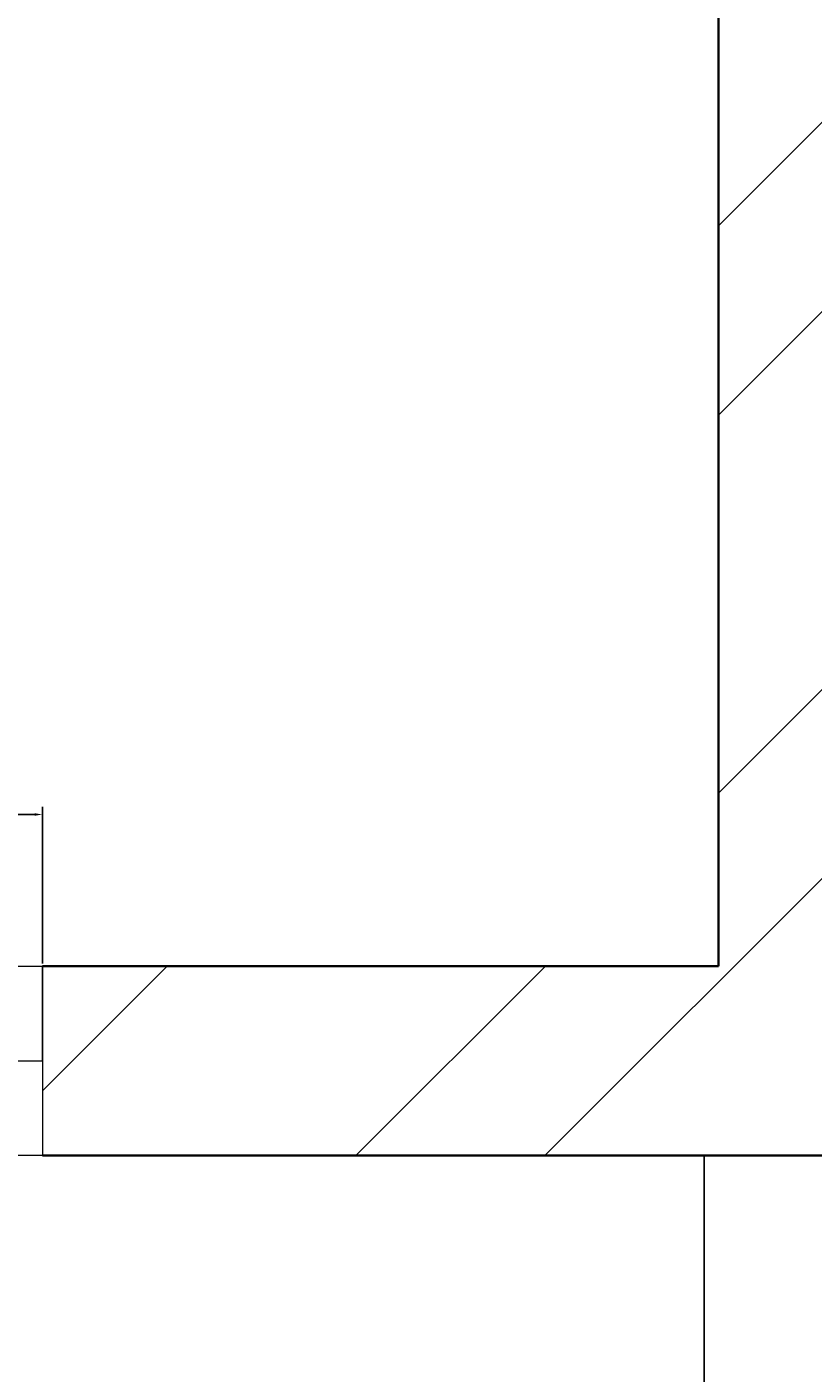
# Model space of a CAD drawing. Units: inches. Extents: x 1885 to 2748, y 783 to 2421.
# Tile 18 of 117: x 2144 to 2163, y 1082 to 1114. Entities that reach past the tile are written whole.
import ezdxf

# ---------------------------------------------------------------- set-up
doc = ezdxf.new("R2010")
doc.units = ezdxf.units.IN
for name, color, linetype, lineweight in [('A-ANNO-DIMS', 2, 'Continuous', 18), ('A-FLOR-BALC', 7, 'Continuous', 25), ('A-GLAZ', 181, 'Continuous', 18), ('A-WALL', 7, 'Continuous', 35)]:
    doc.layers.add(name, color=color, linetype=linetype, lineweight=lineweight)
doc.layers.add('A-WALL-PATT', color=85, linetype='Continuous', lineweight=13, true_color=0x58ba48)
doc.styles.get("Standard").update_dxf_attribs({"font": 'arial.ttf'})
doc.dimstyles.get("Standard").update_dxf_attribs({"dimtxt": 0.18, "dimasz": 0.18, "dimexe": 0.18, "dimexo": 0.0625, "dimgap": 0.09, "dimtad": 0, "dimtih": 1, "dimtoh": 1, "dimdec": 4, "dimzin": 0, "dimdsep": 46, "dimtxsty": 'Standard', "dimcen": 0.09, "dimadec": 0, "dimazin": 0, "dimtfac": 1, "dimtdec": 4, "dimtofl": 0, "dimtmove": 0, "dimatfit": 3, "dimfxl": 1, "dimtolj": 1, "dimtzin": 0, "dimarcsym": 0})

# ---------------------------------------------------------------- blocks, each defined once
blk = doc.blocks.new('WIN-24')
for p, q in [((0.001, 4.496), (0.001, -0.004)), ((0.001, 4.496), (24.001, 4.496)), ((24.001, 2.246), (24.001, 4.496)), ((24.001, 4.496), (24.001, -0.004)), ((0.001, -0.004), (0.001, 2.246)), ((0.001, 2.246), (24.001, 2.246)), ((24.001, -0.004), (0.001, -0.004))]:
    blk.add_line(p, q)
blk = doc.blocks.new('*D23')
at = {"layer": 'A-ANNO-DIMS', "color": 0, "lineweight": -2, "transparency": 16777216}
for p, q in [((2120.221, 1092.068), (2120.221, 1095.786)), ((2144.221, 1092.068), (2144.221, 1095.786)), ((2120.401, 1095.606), (2131.102, 1095.606)), ((2144.041, 1095.606), (2133.339, 1095.606))]:
    blk.add_line(p, q, dxfattribs=at)
at = {"layer": 'A-ANNO-DIMS', "color": 0, "transparency": 16777216}
for points in [[(2120.401, 1095.636), (2120.401, 1095.576), (2120.221, 1095.606)], [(2144.041, 1095.636), (2144.041, 1095.576), (2144.221, 1095.606)]]:
    blk.add_solid(points, dxfattribs=at)
at = {"layer": 'Defpoints', "color": 0, "transparency": 16777216}
for p in [(2144.221, 1095.606), (2120.221, 1092.006), (2144.221, 1092.006)]:
    blk.add_point(p, dxfattribs=at)
at = {"layer": 'A-ANNO-DIMS', "color": 0, "transparency": 16777216, "insert": (2132.221, 1095.606), "char_height": 0.18, "attachment_point": 5}
blk.add_mtext('\\A1;WINDOW 24 TYP.', dxfattribs=at)

msp = doc.modelspace()

# ---------------------------------------------------------------- hatches: boundary and pattern name
at = {"layer": 'A-WALL-PATT'}
h = msp.add_hatch(dxfattribs=at)
h.set_pattern_fill('ANSI32', color=256)
h.paths.add_polyline_path([(2007.772, 2318.006), (1980.774, 2318.006), (1980.774, 2281.215), (1985.274, 2281.215), (1985.274, 2313.506), (2007.772, 2313.506), (2007.772, 2315.756)])
h.paths.add_polyline_path([(2094.324, 2318.006), (2067.772, 2318.006), (2067.772, 2313.506), (2094.324, 2313.506), (2094.324, 2315.756)])
h.paths.add_polyline_path([(2131.367, 2315.756), (2131.367, 2318.006), (2131.189, 2318.006), (2112.609, 2318.006), (2112.609, 2313.506), (2117.274, 2313.506), (2117.274, 2255.201), (2121.774, 2255.201), (2121.774, 2313.506), (2131.367, 2313.506)])
h.paths.add_polyline_path([(2190.512, 2318.006), (2155.367, 2318.006), (2155.367, 2313.506), (2169.774, 2313.506), (2169.774, 2229.506), (2121.774, 2229.506), (2121.774, 2233.451), (2119.524, 2233.451), (2117.274, 2233.451), (2117.274, 2201.101), (2121.774, 2201.101), (2121.774, 2225.006), (2169.774, 2225.006), (2169.774, 2165.006), (2306.274, 2165.006), (2306.274, 2066.006), (2310.774, 2066.006), (2344.274, 2066.006), (2486.274, 2066.006), (2486.274, 1886.006), (2483.02, 1886.006), (2483.02, 1881.506), (2486.274, 1881.506), (2486.274, 1880.678), (2490.774, 1880.678), (2490.774, 2070.506), (2344.274, 2070.506), (2310.774, 2070.506), (2310.774, 2165.006), (2310.774, 2173.636), (2308.524, 2173.636), (2306.274, 2173.636), (2306.274, 2169.506), (2174.274, 2169.506), (2174.274, 2313.506), (2190.512, 2313.506), (2190.512, 2315.756)])
h.paths.add_polyline_path([(1985.274, 2221.215), (1980.774, 2221.215), (1980.774, 2165.006), (1992.774, 2165.006), (1992.774, 2141.927), (1997.274, 2141.927), (1997.274, 2165.006), (2117.274, 2165.006), (2117.274, 2163.126), (2121.774, 2163.126), (2121.774, 2172.734), (2119.524, 2172.734), (2117.274, 2172.734), (2117.274, 2169.506), (1985.274, 2169.506)])
h.paths.add_polyline_path([(1997.274, 2105.927), (1992.774, 2105.927), (1992.774, 2070.506), (2016.774, 2070.506), (2016.774, 2059.123), (2019.024, 2059.123), (2021.274, 2059.123), (2021.274, 2070.506), (2117.274, 2070.506), (2117.274, 2022.506), (2114.423, 2022.506), (2114.423, 2018.006), (2123.627, 2018.006), (2123.627, 2020.256), (2123.627, 2022.506), (2121.774, 2022.506), (2121.774, 2142.587), (2119.524, 2142.587), (2117.274, 2142.587), (2117.274, 2075.006), (1997.274, 2075.006)])
h.paths.add_polyline_path([(2092.029, 2020.256), (2092.029, 2022.506), (2021.274, 2022.506), (2021.274, 2035.123), (2016.774, 2035.123), (2016.774, 2018.006), (2016.774, 1978.784), (2021.274, 1978.784), (2021.274, 2018.006), (2092.029, 2018.006)])
h.paths.add_polyline_path([(2260.938, 2022.506), (2153.105, 2022.506), (2153.105, 2020.256), (2153.105, 2018.006), (2155.274, 2018.006), (2155.274, 1886.006), (2107.629, 1886.006), (2107.629, 1881.506), (2182.911, 1881.506), (2182.911, 1883.756), (2182.911, 1886.006), (2159.774, 1886.006), (2159.774, 2018.006), (2260.938, 2018.006), (2260.938, 2020.256)])
h.paths.add_polyline_path([(2047.629, 1883.756), (2047.629, 1886.006), (2021.274, 1886.006), (2021.274, 1918.784), (2019.024, 1918.784), (2016.774, 1918.784), (2016.774, 1881.506), (2047.629, 1881.506)])
h.paths.add_polyline_path([(2306.361, 1883.756), (2306.361, 1886.006), (2296.274, 1886.006), (2296.274, 1982.006), (2316.535, 1982.006), (2316.535, 1984.256), (2316.535, 1986.506), (2296.274, 1986.506), (2296.274, 2022.506), (2289.276, 2022.506), (2289.276, 2018.006), (2291.774, 2018.006), (2291.774, 1886.006), (2242.911, 1886.006), (2242.911, 1881.506), (2306.361, 1881.506)], flags=17)
h.paths.add_polyline_path([(1985.274, 1843.006), (2021.6, 1843.006), (2021.534, 1845.441), (2021.477, 1847.506), (1980.774, 1847.506), (1980.774, 1809.446), (1985.274, 1809.446)])
h.paths.add_polyline_path([(2131.482, 1845.256), (2131.482, 1847.506), (2081.534, 1847.506), (2081.534, 1843.006), (2117.274, 1843.006), (2117.274, 1784.147), (2119.524, 1784.147), (2121.774, 1784.147), (2121.774, 1843.006), (2131.482, 1843.006)])
h.paths.add_polyline_path([(2203.886, 1847.506), (2155.482, 1847.506), (2155.482, 1843.006), (2169.774, 1843.006), (2169.774, 1759.006), (2121.774, 1759.006), (2121.774, 1761.457), (2117.274, 1761.457), (2117.274, 1730.429), (2121.774, 1730.429), (2121.774, 1754.506), (2177.421, 1754.506), (2177.421, 1756.756), (2177.421, 1759.006), (2174.274, 1759.006), (2174.274, 1843.006), (2203.886, 1843.006)])
h.paths.add_polyline_path([(2335.554, 1845.256), (2335.554, 1847.506), (2239.886, 1847.506), (2239.886, 1843.006), (2306.274, 1843.006), (2306.274, 1759.006), (2199.486, 1759.006), (2199.486, 1754.506), (2310.774, 1754.506), (2310.774, 1843.006), (2335.554, 1843.006)])
h.paths.add_polyline_path([(2348.774, 2022.506), (2344.274, 2022.506), (2344.274, 1986.506), (2341.681, 1986.506), (2341.681, 1982.006), (2344.274, 1982.006), (2344.274, 1886.006), (2330.361, 1886.006), (2330.361, 1881.506), (2361.627, 1881.506), (2361.627, 1883.756), (2361.627, 1886.006), (2348.774, 1886.006)], flags=17)
h.paths.add_polyline_path([(2283.251, 2315.756), (2283.251, 2318.006), (2238.512, 2318.006), (2238.512, 2313.506), (2283.251, 2313.506)], flags=17)
h.paths.add_polyline_path([(2363.274, 2348.006), (2388.677, 2348.006), (2388.677, 2350.256), (2388.677, 2352.506), (2358.774, 2352.506), (2358.774, 2348.006), (2358.774, 2318.006), (2344.481, 2318.006), (2344.481, 2313.506), (2358.774, 2313.506), (2358.774, 2229.506), (2310.774, 2229.506), (2310.774, 2231.952), (2306.274, 2231.952), (2306.274, 2205.611), (2310.774, 2205.611), (2310.774, 2225.006), (2358.774, 2225.006), (2358.774, 2211.506), (2452.329, 2211.506), (2452.329, 2213.756), (2452.329, 2216.006), (2363.274, 2216.006), (2363.274, 2318.006)])
h.paths.add_polyline_path([(2310.774, 2313.506), (2320.481, 2313.506), (2320.481, 2315.756), (2320.481, 2318.006), (2302.728, 2318.006), (2302.728, 2313.506), (2306.274, 2313.506), (2306.274, 2251.076), (2310.774, 2251.076)], flags=17)
h.paths.add_polyline_path([(2490.774, 2352.506), (2486.274, 2352.506), (2448.677, 2352.506), (2448.677, 2348.006), (2486.274, 2348.006), (2486.274, 2318.006), (2486.274, 2216.006), (2481.78, 2216.006), (2481.78, 2211.506), (2486.274, 2211.506), (2486.274, 2165.006), (2493.289, 2165.006), (2493.289, 2167.256), (2493.289, 2169.506), (2490.774, 2169.506), (2490.774, 2313.506), (2494.429, 2313.506), (2494.429, 2318.006), (2490.774, 2318.006)])
h.paths.add_polyline_path([(2534.653, 2318.006), (2515.691, 2318.006), (2515.691, 2313.506), (2534.653, 2313.506), (2534.653, 2315.756)])
h.paths.add_polyline_path([(2618.274, 2318.006), (2594.653, 2318.006), (2594.653, 2313.506), (2613.774, 2313.506), (2613.774, 2281.706), (2618.274, 2281.706)])
h.paths.add_polyline_path([(2618.274, 2221.706), (2613.774, 2221.706), (2613.774, 2169.506), (2554.019, 2169.506), (2554.019, 2165.006), (2613.774, 2165.006), (2613.774, 2152.878), (2618.274, 2152.878)])
h.paths.add_polyline_path([(2618.274, 2128.878), (2616.024, 2128.878), (2613.774, 2128.878), (2613.774, 2117.006), (2529.774, 2117.006), (2529.774, 2165.006), (2532.848, 2165.006), (2532.848, 2169.506), (2522.867, 2169.506), (2522.867, 2165.006), (2525.274, 2165.006), (2525.274, 2117.006), (2525.274, 2112.506), (2525.274, 2108.576), (2529.774, 2108.576), (2529.774, 2112.506), (2613.774, 2112.506), (2613.774, 2080.19), (2618.274, 2080.19)])
h.paths.add_polyline_path([(2618.274, 2044.19), (2616.024, 2044.19), (2613.774, 2044.19), (2613.774, 2015.506), (2529.774, 2015.506), (2529.774, 2088.582), (2527.524, 2088.582), (2525.274, 2088.582), (2525.274, 2011.006), (2613.774, 2011.006), (2613.774, 1956.755), (2618.274, 1956.755)])
h.paths.add_polyline_path([(2618.274, 1881.506), (2618.274, 1896.755), (2613.774, 1896.755), (2613.774, 1881.506), (2613.774, 1847.506), (2592.715, 1847.506), (2592.715, 1843.006), (2613.774, 1843.006), (2613.774, 1765.006), (2613.774, 1760.506), (2609.621, 1760.506), (2609.621, 1756.006), (2613.774, 1756.006), (2613.774, 1660.006), (2608.544, 1660.006), (2608.544, 1655.506), (2613.774, 1655.506), (2613.774, 1508.158), (2618.274, 1508.158)])
h.paths.add_polyline_path([(2565.774, 1843.006), (2568.997, 1843.006), (2568.997, 1847.506), (2490.774, 1847.506), (2490.774, 1849.7), (2488.524, 1849.7), (2486.274, 1849.7), (2486.274, 1847.506), (2477.274, 1847.506), (2477.274, 1838.506), (2477.274, 1821.493), (2486.274, 1821.493), (2486.274, 1838.506), (2561.274, 1838.506), (2561.274, 1765.006), (2486.274, 1765.006), (2486.274, 1786.157), (2477.274, 1786.157), (2477.274, 1765.006), (2477.274, 1756.006), (2486.274, 1756.006), (2565.774, 1756.006), (2585.621, 1756.006), (2585.621, 1758.256), (2585.621, 1760.506), (2565.774, 1760.506), (2565.774, 1765.006)])
h.paths.add_polyline_path([(2486.274, 1651.006), (2561.274, 1651.006), (2561.274, 1567.006), (2486.274, 1567.006), (2486.274, 1591.321), (2477.274, 1591.321), (2477.274, 1567.006), (2477.274, 1558.006), (2477.274, 1555.439), (2481.774, 1555.439), (2481.774, 1558.006), (2568.653, 1558.006), (2568.653, 1560.256), (2568.653, 1562.506), (2565.774, 1562.506), (2565.774, 1655.506), (2584.544, 1655.506), (2584.544, 1657.756), (2584.544, 1660.006), (2565.774, 1660.006), (2486.274, 1660.006), (2477.274, 1660.006), (2477.274, 1651.006), (2477.274, 1632.989), (2486.274, 1632.989)])
h.paths.add_polyline_path([(2449.967, 1883.756), (2449.967, 1886.006), (2421.627, 1886.006), (2421.627, 1881.506), (2449.967, 1881.506)], flags=17)
h.paths.add_polyline_path([(2447.274, 1847.506), (2395.554, 1847.506), (2395.554, 1843.006), (2442.774, 1843.006), (2442.774, 1809.27), (2447.274, 1809.27)])
h.paths.add_polyline_path([(1985.274, 1749.446), (1980.774, 1749.446), (1980.774, 1694.504), (1985.274, 1694.504), (1985.274, 1694.506), (1986.897, 1694.506), (1986.897, 1697.78), (1986.897, 1699.006), (1985.274, 1699.006)])
h.paths.add_polyline_path([(2152.774, 1699.006), (2121.774, 1699.006), (2121.774, 1703.668), (2119.524, 1703.668), (2117.274, 1703.668), (2117.274, 1699.006), (2009.219, 1699.006), (2009.219, 1694.506), (2148.274, 1694.506), (2148.274, 1692.631), (2152.774, 1692.631)])
h.paths.add_polyline_path([(2016.274, 1694.506), (2011.774, 1694.506), (2011.774, 1558.006), (2040.806, 1558.006), (2040.806, 1560.256), (2040.806, 1562.506), (2016.274, 1562.506)])
h.paths.add_polyline_path([(2152.774, 1663.017), (2150.524, 1663.017), (2148.274, 1663.017), (2148.274, 1562.506), (2100.806, 1562.506), (2100.806, 1558.006), (2165.119, 1558.006), (2165.119, 1560.256), (2165.119, 1562.506), (2152.774, 1562.506), (2152.774, 1610.506), (2224.774, 1610.506), (2224.774, 1607.99), (2229.274, 1607.99), (2229.274, 1615.006), (2152.774, 1615.006)])
h.paths.add_polyline_path([(2238.613, 1560.256), (2238.613, 1562.506), (2229.274, 1562.506), (2229.274, 1588.756), (2227.024, 1588.763), (2224.774, 1588.771), (2224.774, 1562.506), (2189.119, 1562.506), (2189.119, 1558.006), (2238.613, 1558.006)])
h.paths.add_polyline_path([(2336.024, 1560.256), (2336.024, 1562.506), (2310.774, 1562.506), (2310.774, 1656.347), (2308.524, 1656.347), (2306.274, 1656.347), (2306.274, 1562.506), (2286.613, 1562.506), (2286.613, 1558.006), (2336.024, 1558.006)])
h.paths.add_polyline_path([(2447.274, 1690.968), (2445.024, 1690.968), (2442.774, 1690.968), (2442.774, 1687.006), (2306.274, 1687.006), (2306.274, 1680.75), (2310.774, 1680.75), (2310.774, 1682.506), (2442.774, 1682.506), (2442.774, 1562.506), (2396.024, 1562.506), (2396.024, 1558.006), (2447.274, 1558.006)])
h.paths.add_polyline_path([(2447.274, 1749.27), (2445.024, 1749.27), (2442.774, 1749.27), (2442.774, 1717.232), (2447.274, 1717.232)])
h.paths.add_polyline_path([(2044.674, 1521.756), (2044.674, 1524.006), (2007.274, 1524.006), (2007.274, 1503.49), (2009.524, 1503.49), (2011.774, 1503.49), (2011.774, 1519.506), (2044.674, 1519.506)])
h.paths.add_polyline_path([(2177.969, 1521.756), (2177.969, 1524.006), (2104.674, 1524.006), (2104.674, 1519.506), (2145.774, 1519.506), (2145.774, 1387.506), (2143.37, 1387.506), (2143.37, 1383.006), (2251.585, 1383.006), (2251.585, 1385.256), (2251.585, 1387.506), (2150.274, 1387.506), (2150.274, 1519.506), (2177.969, 1519.506)])
h.paths.add_polyline_path([(2298.704, 1524.006), (2237.969, 1524.006), (2237.969, 1519.506), (2282.274, 1519.506), (2282.274, 1387.506), (2279.683, 1387.506), (2279.683, 1383.006), (2286.774, 1383.006), (2286.774, 1419.006), (2312.451, 1419.006), (2312.451, 1421.256), (2312.451, 1423.506), (2286.774, 1423.506), (2286.774, 1519.506), (2298.704, 1519.506), (2298.704, 1521.722)], flags=17)
h.paths.add_polyline_path([(2361.897, 1521.756), (2361.897, 1524.006), (2322.704, 1524.006), (2322.704, 1519.506), (2334.774, 1519.506), (2334.774, 1423.506), (2331.93, 1423.506), (2331.93, 1419.006), (2334.774, 1419.006), (2334.774, 1387.506), (2334.774, 1383.228), (2339.274, 1383.228), (2339.274, 1387.506), (2339.274, 1519.506), (2361.897, 1519.506)], flags=17)
h.paths.add_polyline_path([(2447.274, 1521.756), (2447.274, 1524.006), (2421.897, 1524.006), (2421.897, 1519.506), (2447.274, 1519.506)], flags=17)
h.paths.add_polyline_path([(2481.774, 1529.6), (2479.524, 1529.6), (2477.274, 1529.6), (2477.274, 1524.006), (2474.489, 1524.006), (2474.489, 1519.506), (2477.274, 1519.506), (2477.274, 1334.506), (2296.774, 1334.506), (2296.774, 1240.506), (2160.274, 1240.506), (2160.274, 1180.506), (2112.274, 1180.506), (2112.274, 1207.692), (2110.024, 1207.692), (2107.774, 1207.692), (2107.774, 1171.609), (2112.274, 1171.609), (2112.274, 1176.006), (2160.274, 1176.006), (2160.274, 1092.006), (2144.221, 1092.006), (2144.221, 1087.506), (2189.497, 1087.506), (2189.497, 1089.756), (2189.497, 1092.006), (2164.774, 1092.006), (2164.774, 1236.006), (2296.774, 1236.006), (2296.774, 1231.912), (2301.274, 1231.912), (2301.274, 1330.006), (2481.774, 1330.006), (2481.774, 1387.506)])
h.paths.add_polyline_path([(2618.274, 1448.158), (2613.774, 1448.158), (2613.774, 1382.506), (2529.774, 1382.506), (2525.274, 1382.506), (2525.274, 1307.062), (2529.774, 1307.062), (2529.774, 1378.006), (2613.774, 1378.006), (2613.774, 1354.988), (2618.274, 1354.988)])
h.paths.add_polyline_path([(2618.274, 1318.988), (2613.774, 1318.988), (2613.774, 1281.006), (2529.774, 1281.006), (2529.774, 1283.786), (2527.524, 1283.786), (2525.274, 1283.786), (2525.274, 1228.506), (2516.794, 1228.506), (2516.794, 1224.006), (2533.484, 1224.006), (2533.484, 1226.256), (2533.484, 1228.506), (2529.774, 1228.506), (2529.774, 1276.506), (2613.774, 1276.506), (2613.774, 1266.02), (2618.274, 1266.02)])
h.paths.add_polyline_path([(2618.274, 1134.964), (2613.774, 1134.964), (2613.774, 1092.006), (2594.545, 1092.006), (2594.545, 1087.506), (2618.274, 1087.506)])
h.paths.add_polyline_path([(2534.545, 1092.006), (2509.765, 1092.006), (2509.765, 1087.506), (2534.545, 1087.506), (2534.545, 1089.756)])
h.paths.add_polyline_path([(2481.274, 1224.006), (2484.117, 1224.006), (2484.117, 1226.256), (2484.117, 1228.506), (2476.774, 1228.506), (2476.774, 1198.506), (2471.61, 1198.506), (2471.61, 1194.006), (2476.774, 1194.006), (2476.774, 1062.006), (2436.894, 1062.006), (2436.894, 1057.506), (2476.774, 1057.506), (2481.274, 1057.506), (2481.274, 1062.006), (2481.274, 1087.506), (2485.354, 1087.506), (2485.354, 1089.756), (2485.354, 1092.006), (2481.274, 1092.006), (2481.274, 1117.506)])
h.paths.add_polyline_path([(2439.898, 1198.506), (2349.274, 1198.506), (2349.274, 1194.006), (2349.274, 1180.506), (2301.274, 1180.506), (2301.274, 1201.896), (2299.024, 1201.896), (2296.774, 1201.896), (2296.774, 1172.335), (2299.024, 1172.335), (2301.274, 1172.335), (2301.274, 1176.006), (2349.274, 1176.006), (2349.274, 1092.006), (2334.452, 1092.006), (2334.452, 1087.506), (2349.274, 1087.506), (2349.274, 1057.506), (2353.774, 1057.506), (2376.894, 1057.506), (2376.894, 1059.756), (2376.894, 1062.006), (2353.774, 1062.006), (2353.774, 1087.506), (2353.774, 1180.506), (2353.774, 1194.006), (2439.898, 1194.006), (2439.898, 1196.256)])
h.paths.add_polyline_path([(2270.596, 1089.756), (2270.596, 1092.006), (2249.497, 1092.006), (2249.497, 1087.506), (2270.596, 1087.506)], flags=17)
h.paths.add_polyline_path([(2310.452, 1092.006), (2301.274, 1092.006), (2301.274, 1153.292), (2296.774, 1153.292), (2296.774, 1092.006), (2293.786, 1092.006), (2293.786, 1087.506), (2310.452, 1087.506), (2310.452, 1089.756)], flags=17)
h.paths.add_polyline_path([(2112.274, 1150.328), (2110.024, 1150.328), (2107.774, 1150.328), (2107.774, 1092.006), (2104.465, 1092.006), (2104.465, 1087.506), (2120.221, 1087.506), (2120.221, 1089.756), (2120.221, 1092.006), (2112.274, 1092.006)])
h.paths.add_polyline_path([(2082.172, 1092.006), (2058.144, 1092.006), (2058.144, 1087.506), (2082.172, 1087.506), (2082.172, 1089.756)])
h.paths.add_polyline_path([(1975.774, 1145.638), (1971.274, 1145.638), (1971.274, 1087.506), (1980.774, 1087.506), (1998.144, 1087.506), (1998.144, 1089.756), (1998.144, 1092.006), (1985.274, 1092.006), (1975.774, 1092.006)])
h.paths.add_polyline_path([(2112.274, 1244.385), (2110.024, 1244.385), (2107.774, 1244.385), (2107.774, 1240.506), (1992.274, 1240.506), (1992.274, 1271.008), (1987.774, 1271.008), (1987.774, 1240.506), (1980.774, 1240.506), (1975.774, 1240.506), (1971.274, 1240.506), (1971.274, 1205.638), (1975.774, 1205.638), (1975.774, 1236.006), (2107.774, 1236.006), (2107.774, 1233.444), (2112.274, 1233.444), (2112.274, 1236.006)])
h.paths.add_polyline_path([(2112.274, 1383.006), (2114.783, 1383.006), (2114.783, 1385.256), (2114.783, 1387.506), (2102.476, 1387.506), (2102.476, 1383.006), (2107.774, 1383.006), (2107.774, 1335.006), (2011.774, 1335.006), (2011.774, 1349.939), (2007.274, 1349.939), (2007.274, 1335.006), (1987.774, 1335.006), (1987.774, 1330.506), (1987.774, 1307.008), (1992.274, 1307.008), (1992.274, 1330.506), (2007.274, 1330.506), (2107.774, 1330.506), (2107.774, 1264.711), (2112.274, 1264.711)])
h.paths.add_polyline_path([(2077.857, 1387.506), (2011.774, 1387.506), (2011.774, 1390.036), (2009.524, 1390.036), (2007.274, 1390.036), (2007.274, 1373.939), (2011.774, 1373.939), (2011.774, 1383.006), (2077.857, 1383.006)])
h.paths.add_polyline_path([(2011.774, 1443.49), (2007.274, 1443.49), (2007.274, 1410.248), (2011.774, 1410.248)])

# ---------------------------------------------------------------- linework, layer by layer
at = {"layer": 'A-FLOR-BALC'}
msp.add_line((2159.936, 1087.506), (2159.936, 1057.506), dxfattribs=at)
at = {"layer": 'A-WALL'}
for p, q in [((2160.274, 1176.006), (2160.274, 1092.006)), ((2160.274, 1092.006), (2144.221, 1092.006)), ((2189.497, 1087.506), (2144.221, 1087.506))]:
    msp.add_line(p, q, dxfattribs=at)

# ---------------------------------------------------------------- block references
at = {"layer": 'A-GLAZ'}
msp.add_blockref('WIN-24', (2120.22, 1087.51), dxfattribs=at)

# ---------------------------------------------------------------- dimensions: what is measured, and where the dimension line sits
at = {"layer": 'A-ANNO-DIMS'}
dim = msp.add_linear_dim(base=(2144.221, 1095.606), p1=(2120.221, 1092.006), p2=(2144.221, 1092.006), text='WINDOW <> TYP.', dimstyle='Standard', override={"dimdec": 0, "dimlfac": 1, "dimrnd": 0, "dimzin": 0, "dimdsep": 46, "dimlunit": 2}, dxfattribs=at)
dim.commit()
dim.dimension.update_dxf_attribs({"geometry": '*D23', "text_midpoint": (2132.221, 1095.606)})

doc.saveas('drawing.dxf')
